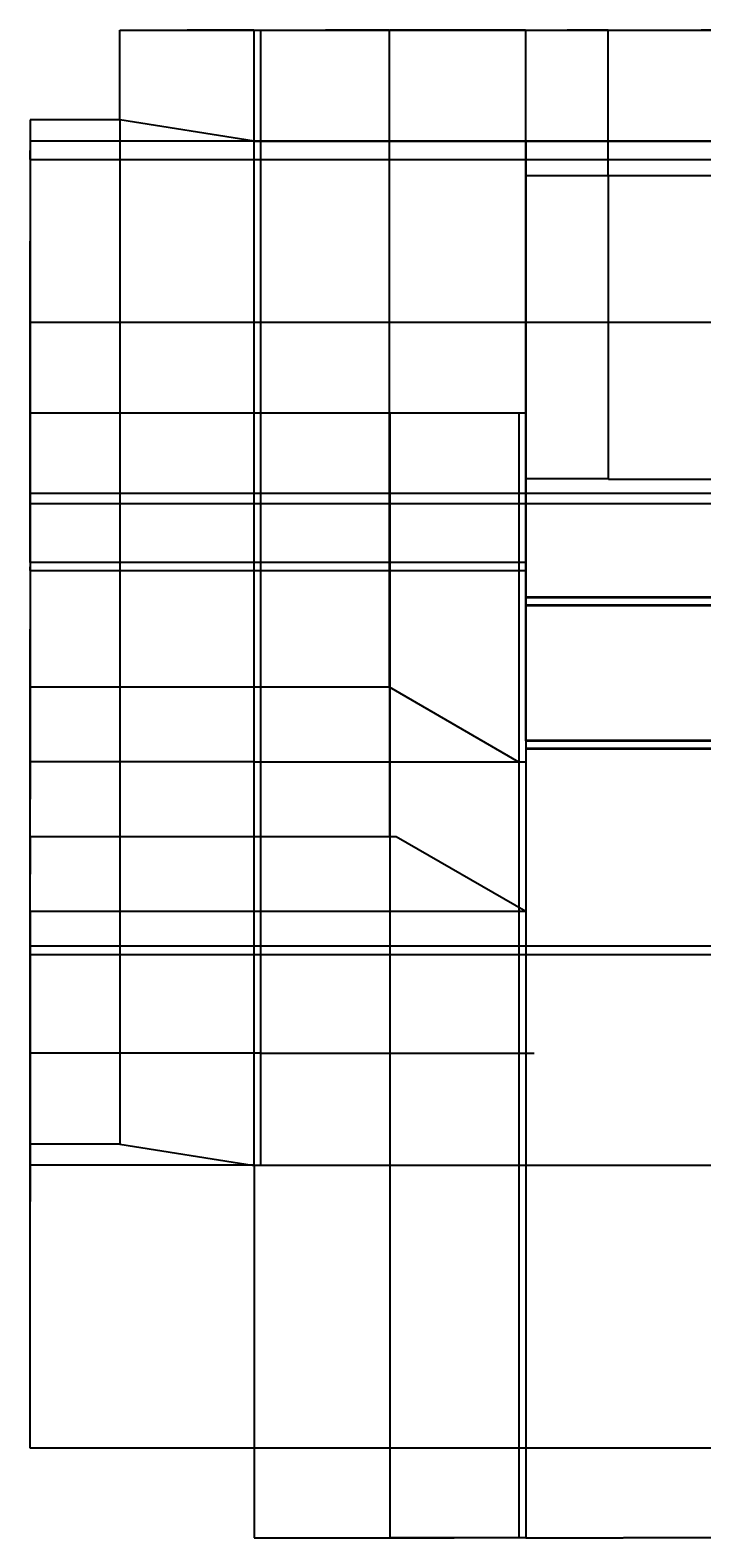
# Model space of a CAD drawing. Units: millimetres. Extents: x 2845 to 7170, y 3531 to 6858.
# Tile 1 of 3: x 2845 to 4328, y 3531 to 6858. Entities that reach past the tile are written whole.
import ezdxf

# ---------------------------------------------------------------- set-up
doc = ezdxf.new("R2010")
doc.units = ezdxf.units.MM
for name, color, linetype, lineweight in [('A-ANNO-DIMS', 2, 'Continuous', 18), ('A-FURN-BASE', 3, 'Continuous', 25), ('A-FURN-CTOP', 6, 'Continuous', 35), ('A-FURN-TALL', 7, 'Continuous', 25)]:
    doc.layers.add(name, color=color, linetype=linetype, lineweight=lineweight)
doc.styles.get("Standard").update_dxf_attribs({"font": 'arial.ttf'})
doc.dimstyles.get("Standard").update_dxf_attribs({"dimtxt": 0.18, "dimasz": 0.18, "dimexe": 0.18, "dimexo": 0.0625, "dimgap": 0.09, "dimtad": 0, "dimtih": 1, "dimtoh": 1, "dimdec": 4, "dimzin": 0, "dimdsep": 46, "dimtxsty": 'Standard', "dimcen": 0.09, "dimadec": 0, "dimazin": 0, "dimtfac": 1, "dimtdec": 4, "dimtofl": 0, "dimtmove": 0, "dimatfit": 3, "dimfxl": 1, "dimtolj": 1, "dimtzin": 0, "dimarcsym": 0})

# ---------------------------------------------------------------- blocks, each defined once
blk = doc.blocks.new('*D1')
at = {"layer": 'A-ANNO-DIMS', "color": 0, "lineweight": -2, "transparency": 16777216}
for p, q in [((3042.6, 6659.7), (2844.7, 6659.7)), ((2844.9, 6659.5), (2844.9, 5194.4)), ((2844.9, 3728.9), (2844.9, 5194)), ((6608, 3728.7), (2844.7, 3728.7))]:
    blk.add_line(p, q, dxfattribs=at)
at = {"layer": 'A-ANNO-DIMS', "color": 0, "transparency": 16777216}
for points in [[(2844.9, 6659.5), (2844.9, 6659.5), (2844.9, 6659.7)], [(2844.9, 3728.9), (2844.9, 3728.9), (2844.9, 3728.7)]]:
    blk.add_solid(points, dxfattribs=at)
at = {"layer": 'Defpoints', "color": 0, "transparency": 16777216}
for p in [(2844.9, 6659.7), (3042.7, 6659.7), (6608.1, 3728.7)]:
    blk.add_point(p, dxfattribs=at)
at = {"layer": 'A-ANNO-DIMS', "color": 0, "transparency": 16777216, "insert": (2844.9, 5194.2), "char_height": 0.18, "attachment_point": 5}
blk.add_mtext('\\A1;2931', dxfattribs=at)
blk = doc.blocks.new('*D2')
at = {"layer": 'A-ANNO-DIMS', "color": 0, "lineweight": -2, "transparency": 16777216}
for p, q in [((3042.7, 6659.8), (3042.7, 6857.7)), ((3042.8, 6857.5), (5006.9, 6857.5)), ((6971.9, 6857.5), (5007.8, 6857.5)), ((6972.1, 4944.1), (6972.1, 6857.7))]:
    blk.add_line(p, q, dxfattribs=at)
at = {"layer": 'A-ANNO-DIMS', "color": 0, "transparency": 16777216}
for points in [[(3042.8, 6857.5), (3042.8, 6857.4), (3042.7, 6857.5)], [(6971.9, 6857.5), (6971.9, 6857.4), (6972.1, 6857.5)]]:
    blk.add_solid(points, dxfattribs=at)
at = {"layer": 'Defpoints', "color": 0, "transparency": 16777216}
for p in [(6972.1, 6857.5), (3042.7, 6659.7), (6972.1, 4944.1)]:
    blk.add_point(p, dxfattribs=at)
at = {"layer": 'A-ANNO-DIMS', "color": 0, "transparency": 16777216, "insert": (5007.4, 6857.5), "char_height": 0.18, "attachment_point": 5}
blk.add_mtext('\\A1;3929.4', dxfattribs=at)
blk = doc.blocks.new('*D3')
at = {"layer": 'A-ANNO-DIMS', "color": 0, "lineweight": -2, "transparency": 16777216}
for p, q in [((3042.7, 6659.8), (3042.7, 6857.7)), ((3042.8, 6857.5), (3190.4, 6857.5)), ((3338.8, 6857.5), (3191.2, 6857.5)), ((3339, 6612.8), (3339, 6857.7))]:
    blk.add_line(p, q, dxfattribs=at)
at = {"layer": 'A-ANNO-DIMS', "color": 0, "transparency": 16777216}
for points in [[(3042.8, 6857.5), (3042.8, 6857.4), (3042.7, 6857.5)], [(3338.8, 6857.5), (3338.8, 6857.4), (3339, 6857.5)]]:
    blk.add_solid(points, dxfattribs=at)
at = {"layer": 'Defpoints', "color": 0, "transparency": 16777216}
for p in [(3339, 6857.5), (3042.7, 6659.7), (3339, 6612.8)]:
    blk.add_point(p, dxfattribs=at)
at = {"layer": 'A-ANNO-DIMS', "color": 0, "transparency": 16777216, "insert": (3190.8, 6857.5), "char_height": 0.18, "attachment_point": 5}
blk.add_mtext('\\A1;296.3', dxfattribs=at)
blk = doc.blocks.new('*D4')
at = {"layer": 'A-ANNO-DIMS', "color": 0, "lineweight": -2, "transparency": 16777216}
for p, q in [((3339, 6612.8), (3339, 6857.7)), ((3339.1, 6857.5), (3638.7, 6857.5)), ((3938.8, 6857.5), (3639.2, 6857.5)), ((3939, 6612.8), (3939, 6857.7))]:
    blk.add_line(p, q, dxfattribs=at)
at = {"layer": 'A-ANNO-DIMS', "color": 0, "transparency": 16777216}
for points in [[(3339.1, 6857.5), (3339.1, 6857.4), (3339, 6857.5)], [(3938.8, 6857.5), (3938.8, 6857.4), (3939, 6857.5)]]:
    blk.add_solid(points, dxfattribs=at)
at = {"layer": 'Defpoints', "color": 0, "transparency": 16777216}
for p in [(3939, 6857.5), (3339, 6612.8), (3939, 6612.8)]:
    blk.add_point(p, dxfattribs=at)
at = {"layer": 'A-ANNO-DIMS', "color": 0, "transparency": 16777216, "insert": (3639, 6857.5), "char_height": 0.18, "attachment_point": 5}
blk.add_mtext('\\A1;600', dxfattribs=at)
blk = doc.blocks.new('*D5')
at = {"layer": 'A-ANNO-DIMS', "color": 0, "lineweight": -2, "transparency": 16777216}
for p, q in [((3939, 6537), (3939, 6857.7)), ((3939.1, 6857.5), (4029.7, 6857.5)), ((4121.2, 6857.5), (4030.6, 6857.5)), ((4121.4, 6537), (4121.4, 6857.7))]:
    blk.add_line(p, q, dxfattribs=at)
at = {"layer": 'A-ANNO-DIMS', "color": 0, "transparency": 16777216}
for points in [[(3939.1, 6857.5), (3939.1, 6857.4), (3939, 6857.5)], [(4121.2, 6857.5), (4121.2, 6857.4), (4121.4, 6857.5)]]:
    blk.add_solid(points, dxfattribs=at)
at = {"layer": 'Defpoints', "color": 0, "transparency": 16777216}
for p in [(4121.4, 6857.5), (3939, 6537), (4121.4, 6537)]:
    blk.add_point(p, dxfattribs=at)
at = {"layer": 'A-ANNO-DIMS', "color": 0, "transparency": 16777216, "insert": (4030.2, 6857.5), "char_height": 0.18, "attachment_point": 5}
blk.add_mtext('\\A1;182.45', dxfattribs=at)
blk = doc.blocks.new('*D6')
at = {"layer": 'A-ANNO-DIMS', "color": 0, "lineweight": -2, "transparency": 16777216}
for p, q in [((4121.4, 6537), (4121.4, 6857.7)), ((4121.6, 6857.5), (4325.9, 6857.5)), ((4531.1, 6857.5), (4326.7, 6857.5)), ((4531.3, 6612.8), (4531.3, 6857.7))]:
    blk.add_line(p, q, dxfattribs=at)
at = {"layer": 'A-ANNO-DIMS', "color": 0, "transparency": 16777216}
for points in [[(4121.6, 6857.5), (4121.6, 6857.4), (4121.4, 6857.5)], [(4531.1, 6857.5), (4531.1, 6857.4), (4531.3, 6857.5)]]:
    blk.add_solid(points, dxfattribs=at)
at = {"layer": 'Defpoints', "color": 0, "transparency": 16777216}
for p in [(4531.3, 6857.5), (4531.3, 6612.8), (4121.4, 6537)]:
    blk.add_point(p, dxfattribs=at)
at = {"layer": 'A-ANNO-DIMS', "color": 0, "transparency": 16777216, "insert": (4326.3, 6857.5), "char_height": 0.18, "attachment_point": 5}
blk.add_mtext('\\A1;409.9', dxfattribs=at)
blk = doc.blocks.new('*D10')
at = {"layer": 'A-ANNO-DIMS', "color": 0, "lineweight": -2, "transparency": 16777216}
for p, q in [((3042.6, 6659.7), (2844.7, 6659.7)), ((2844.9, 6659.5), (2844.9, 5529.9)), ((2844.9, 4399.9), (2844.9, 5529.5)), ((3042.6, 4399.7), (2844.7, 4399.7))]:
    blk.add_line(p, q, dxfattribs=at)
at = {"layer": 'A-ANNO-DIMS', "color": 0, "transparency": 16777216}
for points in [[(2844.9, 6659.5), (2844.9, 6659.5), (2844.9, 6659.7)], [(2844.9, 4399.9), (2844.9, 4399.9), (2844.9, 4399.7)]]:
    blk.add_solid(points, dxfattribs=at)
at = {"layer": 'Defpoints', "color": 0, "transparency": 16777216}
for p in [(2844.9, 6659.7), (3042.7, 6659.7), (3042.7, 4399.7)]:
    blk.add_point(p, dxfattribs=at)
at = {"layer": 'A-ANNO-DIMS', "color": 0, "transparency": 16777216, "insert": (2844.9, 5529.7), "char_height": 0.18, "attachment_point": 5}
blk.add_mtext('\\A1;2260', dxfattribs=at)
blk = doc.blocks.new('*D11')
at = {"layer": 'A-ANNO-DIMS', "color": 0, "lineweight": -2, "transparency": 16777216}
for p, q in [((3042.6, 4399.7), (2844.7, 4399.7)), ((2844.9, 4399.5), (2844.9, 4376.4)), ((2844.9, 4352.9), (2844.9, 4376.1)), ((3338.9, 4352.8), (2844.7, 4352.8))]:
    blk.add_line(p, q, dxfattribs=at)
at = {"layer": 'A-ANNO-DIMS', "color": 0, "transparency": 16777216}
for points in [[(2844.9, 4399.5), (2844.9, 4399.5), (2844.9, 4399.7)], [(2844.9, 4352.9), (2844.9, 4352.9), (2844.9, 4352.8)]]:
    blk.add_solid(points, dxfattribs=at)
at = {"layer": 'Defpoints', "color": 0, "transparency": 16777216}
for p in [(3042.7, 4399.7), (2844.9, 4352.8), (3339, 4352.8)]:
    blk.add_point(p, dxfattribs=at)
at = {"layer": 'A-ANNO-DIMS', "color": 0, "transparency": 16777216, "insert": (2844.9, 4376.2), "char_height": 0.18, "attachment_point": 5}
blk.add_mtext('\\A1;46.96', dxfattribs=at)
blk = doc.blocks.new('*D12')
at = {"layer": 'A-ANNO-DIMS', "color": 0, "lineweight": -2, "transparency": 16777216}
for p, q in [((3354.2, 4600.1), (2844.7, 4600.1)), ((2844.9, 4599.9), (2844.9, 4476.6)), ((2844.9, 4352.9), (2844.9, 4476.2)), ((3338.9, 4352.8), (2844.7, 4352.8))]:
    blk.add_line(p, q, dxfattribs=at)
at = {"layer": 'A-ANNO-DIMS', "color": 0, "transparency": 16777216}
for points in [[(2844.9, 4599.9), (2844.9, 4599.9), (2844.9, 4600.1)], [(2844.9, 4352.9), (2844.9, 4352.9), (2844.9, 4352.8)]]:
    blk.add_solid(points, dxfattribs=at)
at = {"layer": 'Defpoints', "color": 0, "transparency": 16777216}
for p in [(2844.9, 4600.1), (3354.2, 4600.1), (3339, 4352.8)]:
    blk.add_point(p, dxfattribs=at)
at = {"layer": 'A-ANNO-DIMS', "color": 0, "transparency": 16777216, "insert": (2844.9, 4476.4), "char_height": 0.18, "attachment_point": 5}
blk.add_mtext('\\A1;247.3', dxfattribs=at)
blk = doc.blocks.new('*D13')
at = {"layer": 'A-ANNO-DIMS', "color": 0, "lineweight": -2, "transparency": 16777216}
for p, q in [((3338.9, 4912.8), (2844.7, 4912.8)), ((2844.9, 4912.6), (2844.9, 4756.6)), ((2844.9, 4600.3), (2844.9, 4756.2)), ((3354.2, 4600.1), (2844.7, 4600.1))]:
    blk.add_line(p, q, dxfattribs=at)
at = {"layer": 'A-ANNO-DIMS', "color": 0, "transparency": 16777216}
for points in [[(2844.9, 4912.6), (2844.9, 4912.6), (2844.9, 4912.8)], [(2844.9, 4600.3), (2844.9, 4600.3), (2844.9, 4600.1)]]:
    blk.add_solid(points, dxfattribs=at)
at = {"layer": 'Defpoints', "color": 0, "transparency": 16777216}
for p in [(2844.9, 4912.8), (3339, 4912.8), (3354.2, 4600.1)]:
    blk.add_point(p, dxfattribs=at)
at = {"layer": 'A-ANNO-DIMS', "color": 0, "transparency": 16777216, "insert": (2844.9, 4756.4), "char_height": 0.18, "attachment_point": 5}
blk.add_mtext('\\A1;312.7', dxfattribs=at)
blk = doc.blocks.new('*D14')
at = {"layer": 'A-ANNO-DIMS', "color": 0, "lineweight": -2, "transparency": 16777216}
for p, q in [((3354.2, 5077.8), (2844.7, 5077.8)), ((2844.9, 5077.6), (2844.9, 4995.4)), ((2844.9, 4912.9), (2844.9, 4995.1)), ((3338.9, 4912.8), (2844.7, 4912.8))]:
    blk.add_line(p, q, dxfattribs=at)
at = {"layer": 'A-ANNO-DIMS', "color": 0, "transparency": 16777216}
for points in [[(2844.9, 5077.6), (2844.9, 5077.6), (2844.9, 5077.8)], [(2844.9, 4912.9), (2844.9, 4912.9), (2844.9, 4912.8)]]:
    blk.add_solid(points, dxfattribs=at)
at = {"layer": 'Defpoints', "color": 0, "transparency": 16777216}
for p in [(2844.9, 5077.8), (3354.2, 5077.8), (3339, 4912.8)]:
    blk.add_point(p, dxfattribs=at)
at = {"layer": 'A-ANNO-DIMS', "color": 0, "transparency": 16777216, "insert": (2844.9, 4995.3), "char_height": 0.18, "attachment_point": 5}
blk.add_mtext('\\A1;165', dxfattribs=at)
blk = doc.blocks.new('*D15')
at = {"layer": 'A-ANNO-DIMS', "color": 0, "lineweight": -2, "transparency": 16777216}
for p, q in [((3338.9, 5242.8), (2844.7, 5242.8)), ((2844.9, 5242.6), (2844.9, 5160.4)), ((2844.9, 5077.9), (2844.9, 5160.1)), ((3354.2, 5077.8), (2844.7, 5077.8))]:
    blk.add_line(p, q, dxfattribs=at)
at = {"layer": 'A-ANNO-DIMS', "color": 0, "transparency": 16777216}
for points in [[(2844.9, 5242.6), (2844.9, 5242.6), (2844.9, 5242.8)], [(2844.9, 5077.9), (2844.9, 5077.9), (2844.9, 5077.8)]]:
    blk.add_solid(points, dxfattribs=at)
at = {"layer": 'Defpoints', "color": 0, "transparency": 16777216}
for p in [(2844.9, 5242.8), (3339, 5242.8), (3354.2, 5077.8)]:
    blk.add_point(p, dxfattribs=at)
at = {"layer": 'A-ANNO-DIMS', "color": 0, "transparency": 16777216, "insert": (2844.9, 5160.3), "char_height": 0.18, "attachment_point": 5}
blk.add_mtext('\\A1;165', dxfattribs=at)
blk = doc.blocks.new('*D16')
at = {"layer": 'A-ANNO-DIMS', "color": 0, "lineweight": -2, "transparency": 16777216}
for p, q in [((3354.2, 5407.8), (2844.7, 5407.8)), ((2844.9, 5407.6), (2844.9, 5325.4)), ((2844.9, 5242.9), (2844.9, 5325.1)), ((3338.9, 5242.8), (2844.7, 5242.8))]:
    blk.add_line(p, q, dxfattribs=at)
at = {"layer": 'A-ANNO-DIMS', "color": 0, "transparency": 16777216}
for points in [[(2844.9, 5407.6), (2844.9, 5407.6), (2844.9, 5407.8)], [(2844.9, 5242.9), (2844.9, 5242.9), (2844.9, 5242.8)]]:
    blk.add_solid(points, dxfattribs=at)
at = {"layer": 'Defpoints', "color": 0, "transparency": 16777216}
for p in [(2844.9, 5407.8), (3354.2, 5407.8), (3339, 5242.8)]:
    blk.add_point(p, dxfattribs=at)
at = {"layer": 'A-ANNO-DIMS', "color": 0, "transparency": 16777216, "insert": (2844.9, 5325.3), "char_height": 0.18, "attachment_point": 5}
blk.add_mtext('\\A1;165', dxfattribs=at)
blk = doc.blocks.new('*D17')
at = {"layer": 'A-ANNO-DIMS', "color": 0, "lineweight": -2, "transparency": 16777216}
for p, q in [((3338.9, 5664.9), (2844.7, 5664.9)), ((2844.9, 5664.8), (2844.9, 5536.5)), ((2844.9, 5407.9), (2844.9, 5536.2)), ((3354.2, 5407.8), (2844.7, 5407.8))]:
    blk.add_line(p, q, dxfattribs=at)
at = {"layer": 'A-ANNO-DIMS', "color": 0, "transparency": 16777216}
for points in [[(2844.9, 5664.8), (2844.9, 5664.8), (2844.9, 5664.9)], [(2844.9, 5407.9), (2844.9, 5407.9), (2844.9, 5407.8)]]:
    blk.add_solid(points, dxfattribs=at)
at = {"layer": 'Defpoints', "color": 0, "transparency": 16777216}
for p in [(2844.9, 5664.9), (3339, 5664.9), (3354.2, 5407.8)]:
    blk.add_point(p, dxfattribs=at)
at = {"layer": 'A-ANNO-DIMS', "color": 0, "transparency": 16777216, "insert": (2844.9, 5536.3), "char_height": 0.18, "attachment_point": 5}
blk.add_mtext('\\A1;257.2', dxfattribs=at)
blk = doc.blocks.new('*D18')
at = {"layer": 'A-ANNO-DIMS', "color": 0, "lineweight": -2, "transparency": 16777216}
for p, q in [((3338.9, 5682.8), (2844.7, 5682.8)), ((3338.9, 5664.9), (2844.7, 5664.9)), ((2844.9, 5682.6), (2844.9, 5674)), ((2844.9, 5665.1), (2844.9, 5673.7))]:
    blk.add_line(p, q, dxfattribs=at)
at = {"layer": 'A-ANNO-DIMS', "color": 0, "transparency": 16777216}
for points in [[(2844.9, 5682.6), (2844.9, 5682.6), (2844.9, 5682.8)], [(2844.9, 5665.1), (2844.9, 5665.1), (2844.9, 5664.9)]]:
    blk.add_solid(points, dxfattribs=at)
at = {"layer": 'Defpoints', "color": 0, "transparency": 16777216}
for p in [(2844.9, 5682.8), (3339, 5682.8), (3339, 5664.9)]:
    blk.add_point(p, dxfattribs=at)
at = {"layer": 'A-ANNO-DIMS', "color": 0, "transparency": 16777216, "insert": (2844.9, 5673.8), "char_height": 0.18, "attachment_point": 5}
blk.add_mtext('\\A1;17.822', dxfattribs=at)
blk = doc.blocks.new('*D19')
at = {"layer": 'A-ANNO-DIMS', "color": 0, "lineweight": -2, "transparency": 16777216}
for p, q in [((3338.9, 6012.8), (2844.7, 6012.8)), ((2844.9, 6012.6), (2844.9, 5847.9)), ((2844.9, 5682.9), (2844.9, 5847.6)), ((3338.9, 5682.8), (2844.7, 5682.8))]:
    blk.add_line(p, q, dxfattribs=at)
at = {"layer": 'A-ANNO-DIMS', "color": 0, "transparency": 16777216}
for points in [[(2844.9, 6012.6), (2844.9, 6012.6), (2844.9, 6012.8)], [(2844.9, 5682.9), (2844.9, 5682.9), (2844.9, 5682.8)]]:
    blk.add_solid(points, dxfattribs=at)
at = {"layer": 'Defpoints', "color": 0, "transparency": 16777216}
for p in [(2844.9, 6012.8), (3339, 6012.8), (3339, 5682.8)]:
    blk.add_point(p, dxfattribs=at)
at = {"layer": 'A-ANNO-DIMS', "color": 0, "transparency": 16777216, "insert": (2844.9, 5847.8), "char_height": 0.18, "attachment_point": 5}
blk.add_mtext('\\A1;330', dxfattribs=at)
blk = doc.blocks.new('*D20')
at = {"layer": 'A-ANNO-DIMS', "color": 0, "lineweight": -2, "transparency": 16777216}
for p, q in [((3338.9, 6612.8), (2844.7, 6612.8)), ((2844.9, 6612.6), (2844.9, 6312.9)), ((2844.9, 6012.9), (2844.9, 6312.6)), ((3338.9, 6012.8), (2844.7, 6012.8))]:
    blk.add_line(p, q, dxfattribs=at)
at = {"layer": 'A-ANNO-DIMS', "color": 0, "transparency": 16777216}
for points in [[(2844.9, 6612.6), (2844.9, 6612.6), (2844.9, 6612.8)], [(2844.9, 6012.9), (2844.9, 6012.9), (2844.9, 6012.8)]]:
    blk.add_solid(points, dxfattribs=at)
at = {"layer": 'Defpoints', "color": 0, "transparency": 16777216}
for p in [(2844.9, 6612.8), (3339, 6612.8), (3339, 6012.8)]:
    blk.add_point(p, dxfattribs=at)
at = {"layer": 'A-ANNO-DIMS', "color": 0, "transparency": 16777216, "insert": (2844.9, 6312.8), "char_height": 0.18, "attachment_point": 5}
blk.add_mtext('\\A1;600', dxfattribs=at)
blk = doc.blocks.new('*D21')
at = {"layer": 'A-ANNO-DIMS', "color": 0, "lineweight": -2, "transparency": 16777216}
for p, q in [((3354.2, 5407.8), (3354.2, 6857.7)), ((3354.4, 6857.5), (3495.7, 6857.5)), ((3637.8, 6857.5), (3496.5, 6857.5)), ((3638, 5407.8), (3638, 6857.7))]:
    blk.add_line(p, q, dxfattribs=at)
at = {"layer": 'A-ANNO-DIMS', "color": 0, "transparency": 16777216}
for points in [[(3354.4, 6857.5), (3354.4, 6857.4), (3354.2, 6857.5)], [(3637.8, 6857.5), (3637.8, 6857.4), (3638, 6857.5)]]:
    blk.add_solid(points, dxfattribs=at)
at = {"layer": 'Defpoints', "color": 0, "transparency": 16777216}
for p in [(3638, 6857.5), (3354.2, 5407.8), (3638, 5407.8)]:
    blk.add_point(p, dxfattribs=at)
at = {"layer": 'A-ANNO-DIMS', "color": 0, "transparency": 16777216, "insert": (3496.1, 6857.5), "char_height": 0.18, "attachment_point": 5}
blk.add_mtext('\\A1;283.8', dxfattribs=at)
blk = doc.blocks.new('*D22')
at = {"layer": 'A-ANNO-DIMS', "color": 0, "lineweight": -2, "transparency": 16777216}
for p, q in [((3639, 6012.7), (3639, 3530.8)), ((3923.8, 6012.7), (3923.8, 3530.8)), ((3639.1, 3531), (3780.9, 3531)), ((3923.6, 3531), (3781.8, 3531))]:
    blk.add_line(p, q, dxfattribs=at)
at = {"layer": 'A-ANNO-DIMS', "color": 0, "transparency": 16777216}
for points in [[(3639.1, 3531), (3639.1, 3530.9), (3639, 3531)], [(3923.6, 3531), (3923.6, 3530.9), (3923.8, 3531)]]:
    blk.add_solid(points, dxfattribs=at)
at = {"layer": 'Defpoints', "color": 0, "transparency": 16777216}
for p in [(3639, 6012.8), (3923.8, 6012.8), (3923.8, 3531)]:
    blk.add_point(p, dxfattribs=at)
at = {"layer": 'A-ANNO-DIMS', "color": 0, "transparency": 16777216, "insert": (3781.4, 3531), "char_height": 0.18, "attachment_point": 5}
blk.add_mtext('\\A1;284.85', dxfattribs=at)
blk = doc.blocks.new('*D23')
at = {"layer": 'A-ANNO-DIMS', "color": 0, "lineweight": -2, "transparency": 16777216}
for p, q in [((4121.5, 6537), (7170, 6537)), ((7169.8, 6536.8), (7169.8, 6202.3)), ((7169.8, 5867.4), (7169.8, 6201.9)), ((4121.5, 5867.2), (7170, 5867.2))]:
    blk.add_line(p, q, dxfattribs=at)
at = {"layer": 'A-ANNO-DIMS', "color": 0, "transparency": 16777216}
for points in [[(7169.8, 6536.8), (7169.8, 6536.8), (7169.8, 6537)], [(7169.8, 5867.4), (7169.8, 5867.4), (7169.8, 5867.2)]]:
    blk.add_solid(points, dxfattribs=at)
at = {"layer": 'Defpoints', "color": 0, "transparency": 16777216}
for p in [(4121.4, 6537), (7169.8, 6537), (4121.4, 5867.2)]:
    blk.add_point(p, dxfattribs=at)
at = {"layer": 'A-ANNO-DIMS', "color": 0, "transparency": 16777216, "insert": (7169.8, 6202.1), "char_height": 0.18, "attachment_point": 5}
blk.add_mtext('\\A1;669.7', dxfattribs=at)
blk = doc.blocks.new('*D24')
at = {"layer": 'A-ANNO-DIMS', "color": 0, "lineweight": -2, "transparency": 16777216}
for p, q in [((3939, 6612.8), (7170, 6612.8)), ((7169.8, 6612.6), (7169.8, 6575.1)), ((7169.8, 6537.2), (7169.8, 6574.7)), ((4121.5, 6537), (7170, 6537))]:
    blk.add_line(p, q, dxfattribs=at)
at = {"layer": 'A-ANNO-DIMS', "color": 0, "transparency": 16777216}
for points in [[(7169.8, 6612.6), (7169.8, 6612.6), (7169.8, 6612.8)], [(7169.8, 6537.2), (7169.8, 6537.2), (7169.8, 6537)]]:
    blk.add_solid(points, dxfattribs=at)
at = {"layer": 'Defpoints', "color": 0, "transparency": 16777216}
for p in [(3939, 6612.8), (7169.8, 6612.8), (4121.4, 6537)]:
    blk.add_point(p, dxfattribs=at)
at = {"layer": 'A-ANNO-DIMS', "color": 0, "transparency": 16777216, "insert": (7169.8, 6574.9), "char_height": 0.18, "attachment_point": 5}
blk.add_mtext('\\A1;75.77', dxfattribs=at)
blk = doc.blocks.new('*D25')
at = {"layer": 'A-ANNO-DIMS', "color": 0, "lineweight": -2, "transparency": 16777216}
for p, q in [((4531.2, 5835.4), (2844.7, 5835.4)), ((2844.9, 5835.2), (2844.9, 5824.2)), ((2844.9, 5812.9), (2844.9, 5823.9)), ((4531.2, 5812.8), (2844.7, 5812.8))]:
    blk.add_line(p, q, dxfattribs=at)
at = {"layer": 'A-ANNO-DIMS', "color": 0, "transparency": 16777216}
for points in [[(2844.9, 5835.2), (2844.9, 5835.2), (2844.9, 5835.4)], [(2844.9, 5812.9), (2844.9, 5812.9), (2844.9, 5812.8)]]:
    blk.add_solid(points, dxfattribs=at)
at = {"layer": 'Defpoints', "color": 0, "transparency": 16777216}
for p in [(2844.9, 5835.4), (4531.3, 5835.4), (4531.3, 5812.8)]:
    blk.add_point(p, dxfattribs=at)
at = {"layer": 'A-ANNO-DIMS', "color": 0, "transparency": 16777216, "insert": (2844.9, 5824.1), "char_height": 0.18, "attachment_point": 5}
blk.add_mtext('\\A1;22.6', dxfattribs=at)
blk = doc.blocks.new('*D26')
at = {"layer": 'A-ANNO-DIMS', "color": 0, "lineweight": -2, "transparency": 16777216}
for p, q in [((4744.4, 6212.8), (2844.7, 6212.8)), ((2844.9, 6212.6), (2844.9, 6024.2)), ((2844.9, 5835.5), (2844.9, 6023.9)), ((4531.2, 5835.4), (2844.7, 5835.4))]:
    blk.add_line(p, q, dxfattribs=at)
at = {"layer": 'A-ANNO-DIMS', "color": 0, "transparency": 16777216}
for points in [[(2844.9, 6212.6), (2844.9, 6212.6), (2844.9, 6212.8)], [(2844.9, 5835.5), (2844.9, 5835.5), (2844.9, 5835.4)]]:
    blk.add_solid(points, dxfattribs=at)
at = {"layer": 'Defpoints', "color": 0, "transparency": 16777216}
for p in [(2844.9, 6212.8), (4744.4, 6212.8), (4531.3, 5835.4)]:
    blk.add_point(p, dxfattribs=at)
at = {"layer": 'A-ANNO-DIMS', "color": 0, "transparency": 16777216, "insert": (2844.9, 6024.1), "char_height": 0.18, "attachment_point": 5}
blk.add_mtext('\\A1;377.4', dxfattribs=at)
blk = doc.blocks.new('*D27')
at = {"layer": 'A-ANNO-DIMS', "color": 0, "lineweight": -2, "transparency": 16777216}
for p, q in [((4531.2, 6571.7), (2844.7, 6571.7)), ((2844.9, 6571.6), (2844.9, 6392.4)), ((2844.9, 6212.9), (2844.9, 6392.1)), ((4744.4, 6212.8), (2844.7, 6212.8))]:
    blk.add_line(p, q, dxfattribs=at)
at = {"layer": 'A-ANNO-DIMS', "color": 0, "transparency": 16777216}
for points in [[(2844.9, 6571.6), (2844.9, 6571.6), (2844.9, 6571.7)], [(2844.9, 6212.9), (2844.9, 6212.9), (2844.9, 6212.8)]]:
    blk.add_solid(points, dxfattribs=at)
at = {"layer": 'Defpoints', "color": 0, "transparency": 16777216}
for p in [(2844.9, 6571.7), (4531.3, 6571.7), (4744.4, 6212.8)]:
    blk.add_point(p, dxfattribs=at)
at = {"layer": 'A-ANNO-DIMS', "color": 0, "transparency": 16777216, "insert": (2844.9, 6392.2), "char_height": 0.18, "attachment_point": 5}
blk.add_mtext('\\A1;359', dxfattribs=at)
blk = doc.blocks.new('*D28')
at = {"layer": 'A-ANNO-DIMS', "color": 0, "lineweight": -2, "transparency": 16777216}
for p, q in [((4531.2, 6612.8), (2844.7, 6612.8)), ((2844.9, 6612.6), (2844.9, 6592.4)), ((2844.9, 6571.9), (2844.9, 6592.1)), ((4531.2, 6571.7), (2844.7, 6571.7))]:
    blk.add_line(p, q, dxfattribs=at)
at = {"layer": 'A-ANNO-DIMS', "color": 0, "transparency": 16777216}
for points in [[(2844.9, 6612.6), (2844.9, 6612.6), (2844.9, 6612.8)], [(2844.9, 6571.9), (2844.9, 6571.9), (2844.9, 6571.7)]]:
    blk.add_solid(points, dxfattribs=at)
at = {"layer": 'Defpoints', "color": 0, "transparency": 16777216}
for p in [(2844.9, 6612.8), (4531.3, 6612.8), (4531.3, 6571.7)]:
    blk.add_point(p, dxfattribs=at)
at = {"layer": 'A-ANNO-DIMS', "color": 0, "transparency": 16777216, "insert": (2844.9, 6592.2), "char_height": 0.18, "attachment_point": 5}
blk.add_mtext('\\A1;41.03', dxfattribs=at)
blk = doc.blocks.new('*D40')
at = {"layer": 'A-ANNO-DIMS', "color": 0, "lineweight": -2, "transparency": 16777216}
for p, q in [((3939, 5289.6), (7170, 5289.6)), ((3939, 5271.7), (7170, 5271.7)), ((7169.8, 5289.4), (7169.8, 5280.8)), ((7169.8, 5271.9), (7169.8, 5280.5))]:
    blk.add_line(p, q, dxfattribs=at)
at = {"layer": 'A-ANNO-DIMS', "color": 0, "transparency": 16777216}
for points in [[(7169.8, 5289.4), (7169.8, 5289.4), (7169.8, 5289.6)], [(7169.8, 5271.9), (7169.8, 5271.9), (7169.8, 5271.7)]]:
    blk.add_solid(points, dxfattribs=at)
at = {"layer": 'Defpoints', "color": 0, "transparency": 16777216}
for p in [(3939, 5289.6), (3939, 5271.7), (7169.8, 5289.6)]:
    blk.add_point(p, dxfattribs=at)
at = {"layer": 'A-ANNO-DIMS', "color": 0, "transparency": 16777216, "insert": (7169.8, 5280.6), "char_height": 0.18, "attachment_point": 5}
blk.add_mtext('\\A1;17.853', dxfattribs=at)
blk = doc.blocks.new('*D41')
at = {"layer": 'A-ANNO-DIMS', "color": 0, "lineweight": -2, "transparency": 16777216}
for p, q in [((3939, 5588.8), (7170, 5588.8)), ((7169.8, 5588.6), (7169.8, 5439.4)), ((7169.8, 5289.7), (7169.8, 5439)), ((3939, 5289.6), (7170, 5289.6))]:
    blk.add_line(p, q, dxfattribs=at)
at = {"layer": 'A-ANNO-DIMS', "color": 0, "transparency": 16777216}
for points in [[(7169.8, 5588.6), (7169.8, 5588.6), (7169.8, 5588.8)], [(7169.8, 5289.7), (7169.8, 5289.7), (7169.8, 5289.6)]]:
    blk.add_solid(points, dxfattribs=at)
at = {"layer": 'Defpoints', "color": 0, "transparency": 16777216}
for p in [(3939, 5588.8), (7169.8, 5588.8), (3939, 5289.6)]:
    blk.add_point(p, dxfattribs=at)
at = {"layer": 'A-ANNO-DIMS', "color": 0, "transparency": 16777216, "insert": (7169.8, 5439.2), "char_height": 0.18, "attachment_point": 5}
blk.add_mtext('\\A1;299.2', dxfattribs=at)
blk = doc.blocks.new('*D42')
at = {"layer": 'A-ANNO-DIMS', "color": 0, "lineweight": -2, "transparency": 16777216}
for p, q in [((3939, 5606.6), (7170, 5606.6)), ((7169.8, 5606.5), (7169.8, 5597.9)), ((7169.8, 5589), (7169.8, 5597.5)), ((3939, 5588.8), (7170, 5588.8))]:
    blk.add_line(p, q, dxfattribs=at)
at = {"layer": 'A-ANNO-DIMS', "color": 0, "transparency": 16777216}
for points in [[(7169.8, 5606.5), (7169.8, 5606.5), (7169.8, 5606.6)], [(7169.8, 5589), (7169.8, 5589), (7169.8, 5588.8)]]:
    blk.add_solid(points, dxfattribs=at)
at = {"layer": 'Defpoints', "color": 0, "transparency": 16777216}
for p in [(3939, 5606.6), (7169.8, 5606.6), (3939, 5588.8)]:
    blk.add_point(p, dxfattribs=at)
at = {"layer": 'A-ANNO-DIMS', "color": 0, "transparency": 16777216, "insert": (7169.8, 5597.7), "char_height": 0.18, "attachment_point": 5}
blk.add_mtext('\\A1;17.853', dxfattribs=at)
blk = doc.blocks.new('*D43')
at = {"layer": 'A-ANNO-DIMS', "color": 0, "lineweight": -2, "transparency": 16777216}
for p, q in [((3939, 5606.7), (3939, 6857.7)), ((3939.1, 6857.5), (4590.2, 6857.5)), ((5242.1, 6857.5), (4591.1, 6857.5)), ((5242.3, 5606.7), (5242.3, 6857.7))]:
    blk.add_line(p, q, dxfattribs=at)
at = {"layer": 'A-ANNO-DIMS', "color": 0, "transparency": 16777216}
for points in [[(3939.1, 6857.5), (3939.1, 6857.4), (3939, 6857.5)], [(5242.1, 6857.5), (5242.1, 6857.4), (5242.3, 6857.5)]]:
    blk.add_solid(points, dxfattribs=at)
at = {"layer": 'Defpoints', "color": 0, "transparency": 16777216}
for p in [(5242.3, 6857.5), (3939, 5606.6), (5242.3, 5606.6)]:
    blk.add_point(p, dxfattribs=at)
at = {"layer": 'A-ANNO-DIMS', "color": 0, "transparency": 16777216, "insert": (4590.6, 6857.5), "char_height": 0.18, "attachment_point": 5}
blk.add_mtext('\\A1;1303.3', dxfattribs=at)
blk = doc.blocks.new('*D44')
at = {"layer": 'A-ANNO-DIMS', "color": 0, "lineweight": -2, "transparency": 16777216}
for p, q in [((3939, 5289.6), (3939, 6857.7)), ((3939.1, 6857.5), (4701.3, 6857.5)), ((5464.4, 6857.5), (4702.2, 6857.5)), ((5464.6, 5289.6), (5464.6, 6857.7))]:
    blk.add_line(p, q, dxfattribs=at)
at = {"layer": 'A-ANNO-DIMS', "color": 0, "transparency": 16777216}
for points in [[(3939.1, 6857.5), (3939.1, 6857.4), (3939, 6857.5)], [(5464.4, 6857.5), (5464.4, 6857.4), (5464.6, 6857.5)]]:
    blk.add_solid(points, dxfattribs=at)
at = {"layer": 'Defpoints', "color": 0, "transparency": 16777216}
for p in [(5464.6, 6857.5), (3939, 5289.6), (5464.6, 5289.6)]:
    blk.add_point(p, dxfattribs=at)
at = {"layer": 'A-ANNO-DIMS', "color": 0, "transparency": 16777216, "insert": (4701.8, 6857.5), "char_height": 0.18, "attachment_point": 5}
blk.add_mtext('\\A1;1525.6', dxfattribs=at)
blk = doc.blocks.new('*D47')
at = {"layer": 'A-ANNO-DIMS', "color": 0, "lineweight": -2, "transparency": 16777216}
for p, q in [((6607.5, 4817.5), (2844.7, 4817.5)), ((2844.9, 4817.4), (2844.9, 4273.3)), ((2844.9, 3728.9), (2844.9, 4272.9)), ((6608, 3728.7), (2844.7, 3728.7))]:
    blk.add_line(p, q, dxfattribs=at)
at = {"layer": 'A-ANNO-DIMS', "color": 0, "transparency": 16777216}
for points in [[(2844.9, 4817.4), (2844.9, 4817.4), (2844.9, 4817.5)], [(2844.9, 3728.9), (2844.9, 3728.9), (2844.9, 3728.7)]]:
    blk.add_solid(points, dxfattribs=at)
at = {"layer": 'Defpoints', "color": 0, "transparency": 16777216}
for p in [(2844.9, 4817.5), (6607.6, 4817.5), (6608.1, 3728.7)]:
    blk.add_point(p, dxfattribs=at)
at = {"layer": 'A-ANNO-DIMS', "color": 0, "transparency": 16777216, "insert": (2844.9, 4273.1), "char_height": 0.18, "attachment_point": 5}
blk.add_mtext('\\A1;1088.8', dxfattribs=at)
blk = doc.blocks.new('*D48')
at = {"layer": 'A-ANNO-DIMS', "color": 0, "lineweight": -2, "transparency": 16777216}
for p, q in [((6608, 4836.6), (2844.7, 4836.6)), ((2844.9, 4836.4), (2844.9, 4827.2)), ((2844.9, 4817.7), (2844.9, 4826.9)), ((6607.5, 4817.5), (2844.7, 4817.5))]:
    blk.add_line(p, q, dxfattribs=at)
at = {"layer": 'A-ANNO-DIMS', "color": 0, "transparency": 16777216}
for points in [[(2844.9, 4836.4), (2844.9, 4836.4), (2844.9, 4836.6)], [(2844.9, 4817.7), (2844.9, 4817.7), (2844.9, 4817.5)]]:
    blk.add_solid(points, dxfattribs=at)
at = {"layer": 'Defpoints', "color": 0, "transparency": 16777216}
for p in [(2844.9, 4836.6), (6608.1, 4836.6), (6607.6, 4817.5)]:
    blk.add_point(p, dxfattribs=at)
at = {"layer": 'A-ANNO-DIMS', "color": 0, "transparency": 16777216, "insert": (2844.9, 4827.1), "char_height": 0.18, "attachment_point": 5}
blk.add_mtext('\\A1;19.06', dxfattribs=at)
blk = doc.blocks.new('*D52')
at = {"layer": 'A-ANNO-DIMS', "color": 0, "lineweight": -2, "transparency": 16777216}
for p, q in [((3339, 4352.7), (3339, 3530.8)), ((3939, 4352.7), (3939, 3530.8)), ((3339.1, 3531), (3638.7, 3531)), ((3938.8, 3531), (3639.2, 3531))]:
    blk.add_line(p, q, dxfattribs=at)
at = {"layer": 'A-ANNO-DIMS', "color": 0, "transparency": 16777216}
for points in [[(3339.1, 3531), (3339.1, 3530.9), (3339, 3531)], [(3938.8, 3531), (3938.8, 3530.9), (3939, 3531)]]:
    blk.add_solid(points, dxfattribs=at)
at = {"layer": 'Defpoints', "color": 0, "transparency": 16777216}
for p in [(3339, 4352.8), (3939, 4352.8), (3939, 3531)]:
    blk.add_point(p, dxfattribs=at)
at = {"layer": 'A-ANNO-DIMS', "color": 0, "transparency": 16777216, "insert": (3639, 3531), "char_height": 0.18, "attachment_point": 5}
blk.add_mtext('\\A1;600', dxfattribs=at)
blk = doc.blocks.new('*D53')
at = {"layer": 'A-ANNO-DIMS', "color": 0, "lineweight": -2, "transparency": 16777216}
for p, q in [((3939, 4352.7), (3939, 3530.8)), ((4369.7, 4352.7), (4369.7, 3530.8)), ((3939.1, 3531), (4153.9, 3531)), ((4369.5, 3531), (4154.7, 3531))]:
    blk.add_line(p, q, dxfattribs=at)
at = {"layer": 'A-ANNO-DIMS', "color": 0, "transparency": 16777216}
for points in [[(3939.1, 3531), (3939.1, 3530.9), (3939, 3531)], [(4369.5, 3531), (4369.5, 3530.9), (4369.7, 3531)]]:
    blk.add_solid(points, dxfattribs=at)
at = {"layer": 'Defpoints', "color": 0, "transparency": 16777216}
for p in [(3939, 4352.8), (4369.7, 4352.8), (4369.7, 3531)]:
    blk.add_point(p, dxfattribs=at)
at = {"layer": 'A-ANNO-DIMS', "color": 0, "transparency": 16777216, "insert": (4154.3, 3531), "char_height": 0.18, "attachment_point": 5}
blk.add_mtext('\\A1;430.7', dxfattribs=at)

msp = doc.modelspace()

# ---------------------------------------------------------------- linework, layer by layer
at = {"layer": 'A-FURN-BASE', "extrusion": (0, 0, -1)}
msp.add_line((4369.677, 4352.7588), (3938.9578, 4352.7588), dxfattribs=at)
at = {"layer": 'A-FURN-CTOP', "extrusion": (0, 0, -1)}
for points in [[(-3938.9578, 5606.6435), (-5242.2853, 5606.6435), (-6084.9137, 5281.2335), (-6972.0668, 4944.0752), (-6607.6118, 4817.5346), (-5766.7252, 5156.141), (-5461.3127, 5271.7102), (-4164.5775, 5271.7102), (-3938.9578, 5271.7102)], [(-3938.9578, 5588.7906), (-5238.9578, 5588.7906), (-6078.5267, 5264.5621), (-6919.8193, 4944.8329), (-6608.0753, 4836.5939), (-5773.2194, 5172.7719), (-5464.5775, 5289.563), (-4164.5775, 5289.563), (-3938.9578, 5289.563)]]:
    msp.add_lwpolyline(points, dxfattribs=at)
at = {"layer": 'A-FURN-TALL'}
for p, q in [((3338.9578, 6612.7588), (3938.9578, 6612.7588)), ((3938.9578, 6612.7588), (3938.9578, 6012.7588)), ((3938.9578, 6012.7588), (3338.9578, 6012.7588)), ((3923.806, 6012.7588), (3923.806, 5682.7588)), ((3938.9578, 6012.7588), (3938.9578, 5682.7588)), ((3938.9578, 5682.7588), (3338.9578, 5682.7588)), ((3938.9578, 5664.9364), (3338.9578, 5664.9364)), ((3923.806, 5682.7588), (3923.806, 5242.7588)), ((3938.9578, 5682.7588), (3938.9578, 5242.7588)), ((3938.9578, 5242.7588), (3338.9578, 5242.7588)), ((3938.9578, 5242.7588), (3938.9578, 4912.7588)), ((3938.9578, 4912.7588), (3338.9578, 4912.7588)), ((3938.9578, 4912.7588), (3938.9578, 4352.7588)), ((3938.9578, 4352.7588), (3338.9578, 4352.7588))]:
    msp.add_line(p, q, dxfattribs=at)
at = {"layer": 'A-FURN-TALL', "extrusion": (0, 0, -1)}
for p, q in [((3638.0176, 5407.7588), (3638.9578, 6012.7588)), ((3653.1694, 5077.7588), (3354.2304, 5077.7588)), ((3938.9578, 4912.7588), (3653.1694, 5077.7588)), ((3354.2304, 4600.078), (3957.8261, 4600.078))]:
    msp.add_line(p, q, dxfattribs=at)
at = {"layer": 'A-FURN-TALL'}
for points in [[(3338.9578, 6612.7588), (3042.6566, 6659.7224), (3042.6566, 4399.7224), (3338.9578, 4352.7588)], [(3338.9578, 4352.7588), (3338.9578, 6612.7588)], [(3354.2304, 4352.7588), (3354.2304, 6612.7588)], [(3938.9578, 6536.9844), (4121.4047, 6536.9844), (4121.4047, 5867.2425), (3938.9578, 5867.2425)]]:
    msp.add_lwpolyline(points, dxfattribs=at)
at = {"layer": 'A-FURN-TALL', "extrusion": (0, 0, -1)}
for points in [[(-3923.806, 5242.7588), (-3638.0176, 5407.7588), (-3354.2304, 5407.7588)], [(-3638.0176, 5407.7588), (-3638.0176, 5077.7588)]]:
    msp.add_lwpolyline(points, dxfattribs=at)

# ---------------------------------------------------------------- dimensions: what is measured, and where the dimension line sits
at = {"layer": 'A-ANNO-DIMS'}
for base, p1, p2, override, picture, middle in [((6972.0668, 6857.4724), (3042.6566, 6659.7224), (6972.0668, 4944.0752), {"dimdec": 1, "dimlfac": 1, "dimrnd": 0, "dimzin": 0, "dimdsep": 46, "dimlunit": 2}, '*D2', (5007.3617, 6857.4724)), ((3338.9578, 6857.4724), (3042.6566, 6659.7224), (3338.9578, 6612.7588), {"dimdec": 1, "dimlfac": 1, "dimrnd": 0, "dimzin": 0, "dimdsep": 46, "dimlunit": 2}, '*D3', (3190.8072, 6857.4724)), ((3938.9578, 6857.4724), (3338.9578, 6612.7588), (3938.9578, 6612.7588), {"dimdec": 0, "dimlfac": 1, "dimrnd": 0, "dimzin": 0, "dimdsep": 46, "dimlunit": 2}, '*D4', (3638.9578, 6857.4724)), ((3638.0176, 6857.4724), (3354.2304, 5407.7588), (3638.0176, 5407.7588), {"dimdec": 1, "dimlfac": 1, "dimrnd": 0, "dimzin": 0, "dimdsep": 46, "dimlunit": 2}, '*D21', (3496.124, 6857.4724)), ((4121.4047, 6857.4724), (3938.9578, 6536.9844), (4121.4047, 6536.9844), {"dimdec": 2, "dimlfac": 1, "dimrnd": 0, "dimzin": 0, "dimdsep": 46, "dimlunit": 2}, '*D5', (4030.1812, 6857.4724)), ((5242.2853, 6857.4724), (3938.9578, 5606.6435), (5242.2853, 5606.6435), {"dimdec": 1, "dimlfac": 1, "dimrnd": 0, "dimzin": 0, "dimdsep": 46, "dimlunit": 2}, '*D43', (4590.6216, 6857.4724)), ((5464.5775, 6857.4724), (3938.9578, 5289.563), (5464.5775, 5289.563), {"dimdec": 1, "dimlfac": 1, "dimrnd": 0, "dimzin": 0, "dimdsep": 46, "dimlunit": 2}, '*D44', (4701.7677, 6857.4724)), ((4531.2682, 6857.4724), (4121.4047, 6536.9844), (4531.2682, 6612.7588), {"dimdec": 1, "dimlfac": 1, "dimrnd": 0, "dimzin": 0, "dimdsep": 46, "dimlunit": 2}, '*D6', (4326.3364, 6857.4724)), ((3923.806, 3530.9704), (3638.9578, 6012.7588), (3923.806, 6012.7588), {"dimdec": 2, "dimlfac": 1, "dimrnd": 0, "dimzin": 0, "dimdsep": 46, "dimlunit": 2}, '*D22', (3781.3819, 3530.9704)), ((3938.9578, 3530.9704), (3338.9578, 4352.7588), (3938.9578, 4352.7588), {"dimdec": 0, "dimlfac": 1, "dimrnd": 0, "dimzin": 0, "dimdsep": 46, "dimlunit": 2}, '*D52', (3638.9578, 3530.9704)), ((4369.677, 3530.9704), (3938.9578, 4352.7588), (4369.677, 4352.7588), {"dimdec": 1, "dimlfac": 1, "dimrnd": 0, "dimzin": 0, "dimdsep": 46, "dimlunit": 2}, '*D53', (4154.3174, 3530.9704))]:
    dim = msp.add_linear_dim(base=base, p1=p1, p2=p2, dimstyle='Standard', override=override, dxfattribs=at)
    dim.commit()
    dim.dimension.update_dxf_attribs({"geometry": picture, "text_midpoint": middle})
for base, p1, p2, override, picture, middle in [((2844.9066, 6659.7224), (6608.0753, 3728.7204), (3042.6566, 6659.7224), {"dimdec": 0, "dimlfac": 1, "dimrnd": 0, "dimzin": 0, "dimdsep": 46, "dimlunit": 2}, '*D1', (2844.9066, 5194.2214)), ((2844.9066, 6659.7224), (3042.6566, 4399.7224), (3042.6566, 6659.7224), {"dimdec": 0, "dimlfac": 1, "dimrnd": 0, "dimzin": 0, "dimdsep": 46, "dimlunit": 2}, '*D10', (2844.9066, 5529.7224)), ((2844.9066, 6612.7588), (4531.2682, 6571.7311), (4531.2682, 6612.7588), {"dimdec": 2, "dimlfac": 1, "dimrnd": 0, "dimzin": 0, "dimdsep": 46, "dimlunit": 2}, '*D28', (2844.9066, 6592.245)), ((2844.9066, 6612.7588), (3338.9578, 6012.7588), (3338.9578, 6612.7588), {"dimdec": 0, "dimlfac": 1, "dimrnd": 0, "dimzin": 0, "dimdsep": 46, "dimlunit": 2}, '*D20', (2844.9066, 6312.7588)), ((7169.8168, 6612.7588), (4121.4047, 6536.9844), (3938.9578, 6612.7588), {"dimdec": 2, "dimlfac": 1, "dimrnd": 0, "dimzin": 0, "dimdsep": 46, "dimlunit": 2}, '*D24', (7169.8168, 6574.8716)), ((2844.9066, 6571.7311), (4744.4359, 6212.7588), (4531.2682, 6571.7311), {"dimdec": 0, "dimlfac": 1, "dimrnd": 0, "dimzin": 0, "dimdsep": 46, "dimlunit": 2}, '*D27', (2844.9066, 6392.245)), ((7169.8168, 6536.9844), (4121.4047, 5867.2425), (4121.4047, 6536.9844), {"dimdec": 1, "dimlfac": 1, "dimrnd": 0, "dimzin": 0, "dimdsep": 46, "dimlunit": 2}, '*D23', (7169.8168, 6202.1134)), ((2844.9066, 6212.7588), (4531.2682, 5835.359), (4744.4359, 6212.7588), {"dimdec": 1, "dimlfac": 1, "dimrnd": 0, "dimzin": 0, "dimdsep": 46, "dimlunit": 2}, '*D26', (2844.9066, 6024.0589)), ((2844.9066, 6012.7588), (3338.9578, 5682.7588), (3338.9578, 6012.7588), {"dimdec": 0, "dimlfac": 1, "dimrnd": 0, "dimzin": 0, "dimdsep": 46, "dimlunit": 2}, '*D19', (2844.9066, 5847.7588)), ((2844.9066, 5835.359), (4531.2682, 5812.7588), (4531.2682, 5835.359), {"dimdec": 1, "dimlfac": 1, "dimrnd": 0, "dimzin": 0, "dimdsep": 46, "dimlunit": 2}, '*D25', (2844.9066, 5824.0589)), ((2844.9066, 5682.7588), (3338.9578, 5664.9364), (3338.9578, 5682.7588), {"dimdec": 3, "dimlfac": 1, "dimrnd": 0, "dimzin": 0, "dimdsep": 46, "dimlunit": 2}, '*D18', (2844.9066, 5673.8476)), ((2844.9066, 5664.9364), (3354.2304, 5407.7588), (3338.9578, 5664.9364), {"dimdec": 1, "dimlfac": 1, "dimrnd": 0, "dimzin": 0, "dimdsep": 46, "dimlunit": 2}, '*D17', (2844.9066, 5536.3476)), ((7169.8168, 5606.6435), (3938.9578, 5588.7906), (3938.9578, 5606.6435), {"dimdec": 3, "dimlfac": 1, "dimrnd": 0, "dimzin": 0, "dimdsep": 46, "dimlunit": 2}, '*D42', (7169.8168, 5597.7171)), ((7169.8168, 5588.7906), (3938.9578, 5289.563), (3938.9578, 5588.7906), {"dimdec": 1, "dimlfac": 1, "dimrnd": 0, "dimzin": 0, "dimdsep": 46, "dimlunit": 2}, '*D41', (7169.8168, 5439.1768)), ((2844.9066, 5407.7588), (3338.9578, 5242.7588), (3354.2304, 5407.7588), {"dimdec": 0, "dimlfac": 1, "dimrnd": 0, "dimzin": 0, "dimdsep": 46, "dimlunit": 2}, '*D16', (2844.9066, 5325.2588)), ((7169.8168, 5289.563), (3938.9578, 5271.7102), (3938.9578, 5289.563), {"dimdec": 3, "dimlfac": 1, "dimrnd": 0, "dimzin": 0, "dimdsep": 46, "dimlunit": 2}, '*D40', (7169.8168, 5280.6366)), ((2844.9066, 5242.7588), (3354.2304, 5077.7588), (3338.9578, 5242.7588), {"dimdec": 0, "dimlfac": 1, "dimrnd": 0, "dimzin": 0, "dimdsep": 46, "dimlunit": 2}, '*D15', (2844.9066, 5160.2588)), ((2844.9066, 5077.7588), (3338.9578, 4912.7588), (3354.2304, 5077.7588), {"dimdec": 0, "dimlfac": 1, "dimrnd": 0, "dimzin": 0, "dimdsep": 46, "dimlunit": 2}, '*D14', (2844.9066, 4995.2588)), ((2844.9066, 4912.7588), (3354.2304, 4600.078), (3338.9578, 4912.7588), {"dimdec": 1, "dimlfac": 1, "dimrnd": 0, "dimzin": 0, "dimdsep": 46, "dimlunit": 2}, '*D13', (2844.9066, 4756.4184)), ((2844.9066, 4836.5939), (6607.6118, 4817.5346), (6608.0753, 4836.5939), {"dimdec": 2, "dimlfac": 1, "dimrnd": 0, "dimzin": 0, "dimdsep": 46, "dimlunit": 2}, '*D48', (2844.9066, 4827.0643)), ((2844.9066, 4817.5346), (6608.0753, 3728.7204), (6607.6118, 4817.5346), {"dimdec": 1, "dimlfac": 1, "dimrnd": 0, "dimzin": 0, "dimdsep": 46, "dimlunit": 2}, '*D47', (2844.9066, 4273.1275)), ((2844.9066, 4600.078), (3338.9578, 4352.7588), (3354.2304, 4600.078), {"dimdec": 1, "dimlfac": 1, "dimrnd": 0, "dimzin": 0, "dimdsep": 46, "dimlunit": 2}, '*D12', (2844.9066, 4476.4184)), ((2844.9066, 4352.7588), (3042.6566, 4399.7224), (3338.9578, 4352.7588), {"dimdec": 2, "dimlfac": 1, "dimrnd": 0, "dimzin": 0, "dimdsep": 46, "dimlunit": 2}, '*D11', (2844.9066, 4376.2406))]:
    dim = msp.add_linear_dim(base=base, p1=p1, p2=p2, angle=90, dimstyle='Standard', override=override, dxfattribs=at)
    dim.commit()
    dim.dimension.update_dxf_attribs({"geometry": picture, "text_midpoint": middle})

doc.saveas('drawing.dxf')
